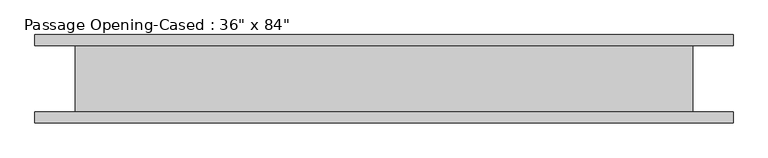
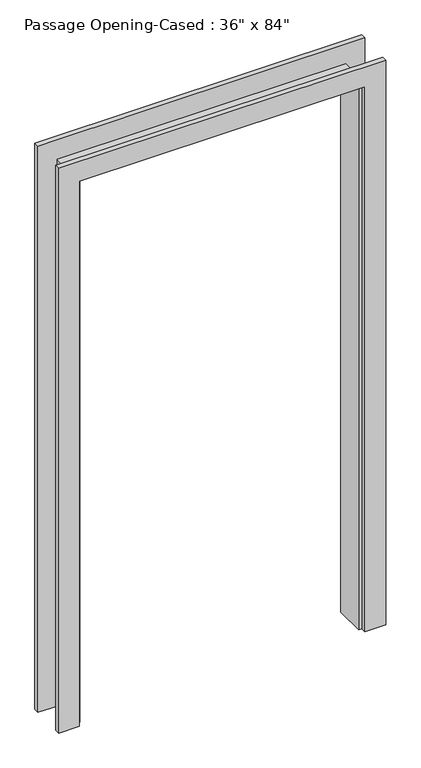
"""IFC4 building model written with IfcOpenShell, lengths in millimetres: proxy geometry."""

from ifc_helpers import new_model, si_unit, frame, origin, place, context, project, spatial, polyline, outline, extrude, faceted_brep, source, transform, mapped, element, save


def proxy_bc9927fa(model_context):
    return source(origin(), model_context, "Body", "SolidModel", [
        faceted_brep([(506.1613433, 57.15, 0.0), (525.2113433, 57.15, 0.0), (525.2113433, -57.15, 0.0), (506.1613433, -57.15, 0.0), (506.1613433, 57.15, 2114.55), (525.2113433, 57.15, 2133.6), (525.2113433, -57.15, 2133.6), (506.1613433, -57.15, 2114.55), (-522.5386567, 57.15, 2114.55), (-541.5886567, 57.15, 2133.6), (-541.5886567, -57.15, 2133.6), (-522.5386567, -57.15, 2114.55), (-522.5386567, 57.15, 0.0), (-522.5386567, -57.15, 0.0), (-541.5886567, -57.15, 0.0), (-541.5886567, 57.15, 0.0)], [[[0, 1, 2, 3]], [[1, 0, 4, 5]], [[2, 1, 5, 6]], [[3, 2, 6, 7]], [[0, 3, 7, 4]], [[5, 4, 8, 9]], [[6, 5, 9, 10]], [[7, 6, 10, 11]], [[4, 7, 11, 8]], [[12, 13, 14, 15]], [[9, 8, 12, 15]], [[10, 9, 15, 14]], [[11, 10, 14, 13]], [[8, 11, 13, 12]]]),
        extrude(outline(polyline([(0.0, 595.0613433), (2209.8, 595.0613433), (2209.8, -611.4386567), (0.0, -611.4386567), (0.0, -535.2386567), (2127.25, -535.2386567), (2127.25, 518.8613433), (0.0, 518.8613433), (0.0, 595.0613433)])), frame((0.0, 57.15, 0.0), z_axis=(0.0, 1.0, 0.0), x_axis=(0.0, 0.0, 1.0)), (0.0, 0.0, 1.0), 19.05),
        extrude(outline(polyline([(0.0, -535.2386567), (2127.25, -535.2386567), (2127.25, 518.8613433), (0.0, 518.8613433), (0.0, 595.0613433), (2203.45, 595.0613433), (2203.45, -611.4386567), (0.0, -611.4386567), (0.0, -535.2386567)])), frame((0.0, -76.2, 0.0), z_axis=(0.0, 1.0, 0.0), x_axis=(0.0, 0.0, 1.0)), (0.0, 0.0, 1.0), 19.05),
    ])


if __name__ == "__main__":
    model = new_model("IFC4")
    model_context = context("Model", 3, world=origin())
    ifc_project = project(units=[si_unit("LENGTHUNIT", "METRE", prefix="MILLI")], contexts=[model_context])
    site = spatial("IfcSite", under=ifc_project)
    building = spatial("IfcBuilding", under=site)
    placement = place(None, origin())
    proxy_shape = proxy_bc9927fa(model_context)
    element("IfcBuildingElementProxy", 1, Name="Passage Opening-Cased : 36\" x 84\"", ObjectType="Passage Opening-Cased : 36\" x 84\"", at=placement, inside=building, context=model_context, shape_type="MappedRepresentation", body=[
        mapped(proxy_shape, transform((0.0, 0.0, 0.0), x_axis=(1.0, 0.0, 0.0), y_axis=(0.0, 1.0, 0.0), z_axis=(0.0, 0.0, 1.0))),
    ])
    save(model, "model.ifc")

# Revit data of these elements
# Type "Passage Opening-Cased : 36\" x 84\""
#   Height = 7' - 0"
#   Trim Thickness = 0' - 0 3/4"
#   Trim Width = 0' - 3"
#   Width = 3' - 6"
#   Frame Material = Door - Frame
#   Default Elevation = 0
# Element 1 (IfcBuildingElementProxy, "Passage Opening-Cased : 36\" x 84\"")
#   Materials on its faces: "Door - Frame"
# Materials
#   "Door - Frame": colour RGB 118 70 51, transparency 0, Cost = 0
